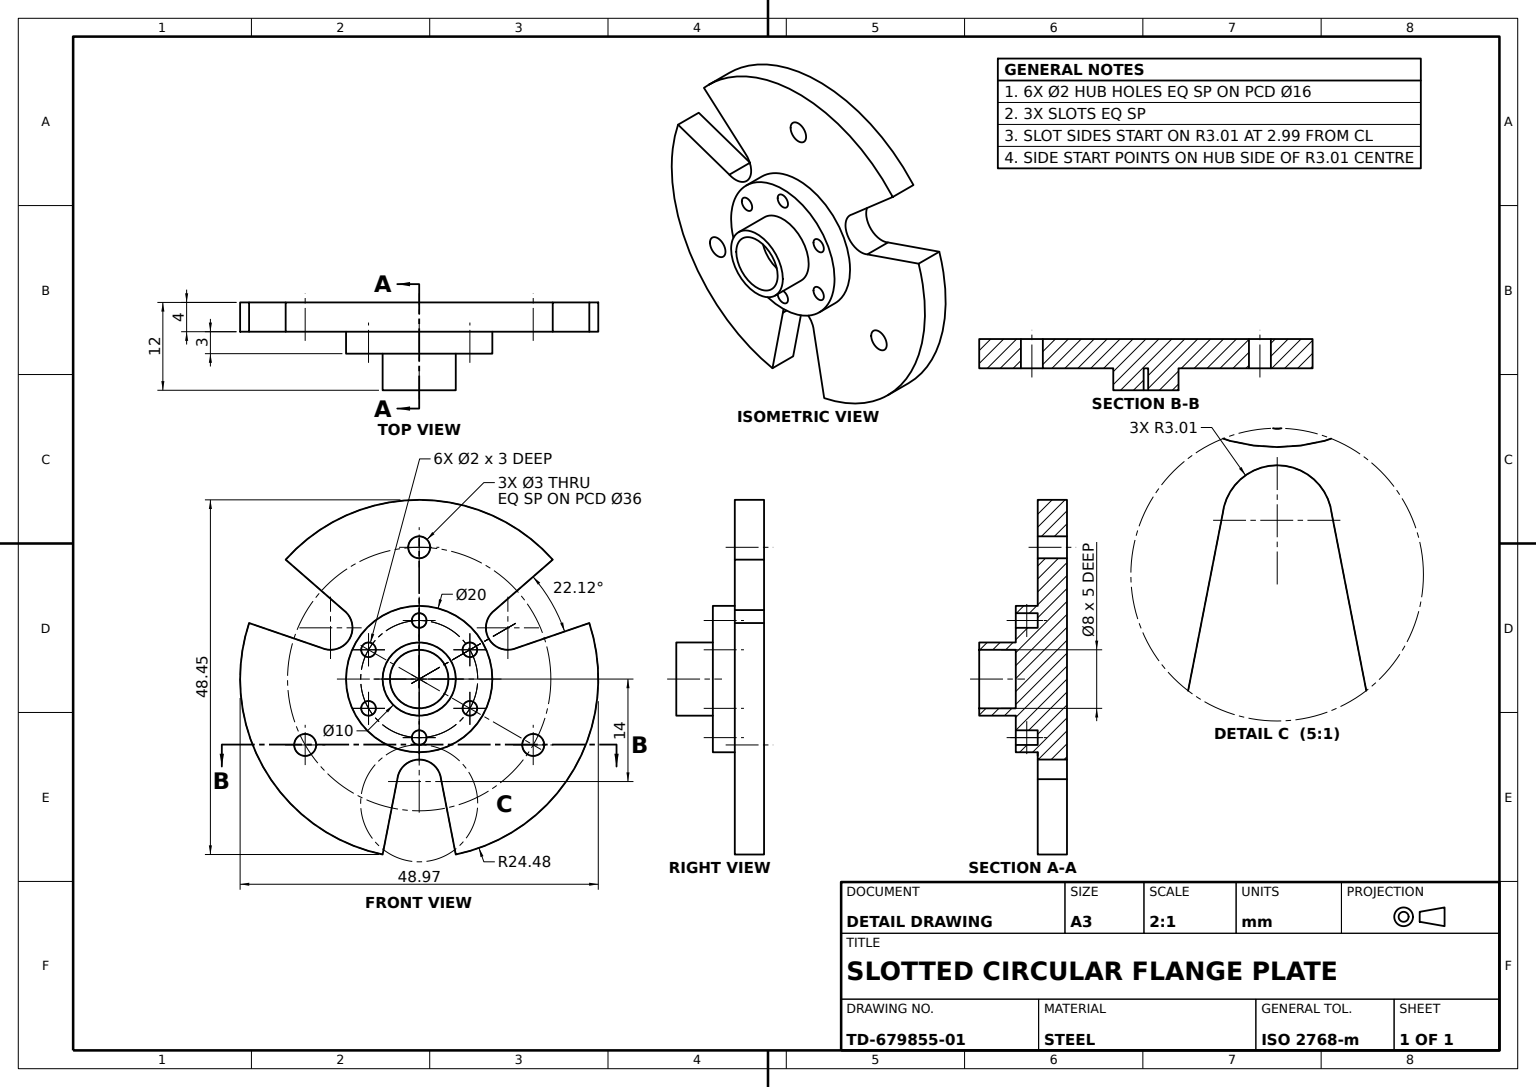
SolidWorks part; units mm, degrees
material "Plain Carbon Steel"
ref_plane "Front Plane" through (0, 0, 0) normal (0, 0, 1) x (1, 0, 0)
ref_plane "Top Plane" through (0, 0, 0) normal (0, 1, 0) x (1, 0, 0)
ref_plane "Right Plane" through (0, 0, 0) normal (1, 0, 0) x (0, 0, -1)
sketch "Flange Plate Sketch" plane through (0, 0, 0) normal (0, 0, 1) x (1, 0, 0)
  line L0 (0, 0) -> (0, 24.4841) construction
  line L1 (0, -17) -> (0, -28.4926) construction
  line L2 (-2.9887, -13.6773) -> (-5, -23.9681)
  line L3 (2.9887, -13.6773) -> (5, -23.9681)
  line L4 (-10.3505, 9.4269) -> (-18.257, 16.3142)
  line L5 (-13.3392, 4.2503) -> (-23.257, 7.6539)
  line L6 (13.3392, 4.2503) -> (23.257, 7.6539)
  line L7 (10.3505, 9.4269) -> (18.257, 16.3142)
  arc A0 (5, -23.9681) -> (23.257, 7.6539) centre (0, 0) ccw
  arc A2 (2.9887, -13.6773) -> (-2.9887, -13.6773) centre (0, -14) ccw
  arc A3 (-13.3392, 4.2503) -> (-10.3505, 9.4269) centre (-12.1244, 7) ccw
  arc A4 (10.3505, 9.4269) -> (13.3392, 4.2503) centre (12.1244, 7) ccw
  arc A5 (-23.257, 7.6539) -> (-5, -23.9681) centre (0, 0) ccw
  arc A6 (18.257, 16.3142) -> (-18.257, 16.3142) centre (0, 0) ccw
  point P13 (0, 0)
  point P25 (0, 0)
  dimension "D1" = 3
  dimension "D4" = 24.4841
  dimension "D5" = 3.0061
  dimension "D6" = 2.9887
  dimension "D7" = 10.3505
  dimension "D2" = 3
  dimension "D3" = 10
extrude "Flange Plate 4mm" add sketch "Flange Plate Sketch" along normal blind 4
sketch "Outer Holes Sketch" plane through (0, 0, 0) normal (0, 0, 1) x (1, 0, 0)
  circle A0 centre (0, 0) radius 18 construction
  circle A1 centre (0, 18) radius 1.5
  circle A2 centre (15.5885, -9) radius 1.5
  circle A3 centre (-15.5885, -9) radius 1.5
  point P11 (0, 0)
  dimension "D1" = 3
  dimension "D2" = 3
  dimension "D5" = 36
extrude "Outer Holes 3x" cut sketch "Outer Holes Sketch" along normal through all
sketch "Hub Sketch" plane through (0, 0, 0) normal (0, 0, 1) x (1, 0, 0)
  circle A0 centre (0, 0) radius 10
  dimension "D1" = 20
extrude "Raised Hub" add sketch "Hub Sketch" along normal blind 7
sketch "Hub Holes Sketch" plane through (0, 0, 7) normal (0, 0, 1) x (1, 0, 0)
  circle A0 centre (0, 0) radius 8 construction
  circle A1 centre (0, 8) radius 1
  circle A2 centre (0.0005, 0.0009) radius 8 construction
  circle A3 centre (6.9287, 4.0009) radius 1
  circle A4 centre (0.0015, 0.0009) radius 8 construction
  circle A5 centre (6.9297, -3.9991) radius 1
  circle A6 centre (0.002, 0) radius 8 construction
  circle A7 centre (0.002, -8) radius 1
  circle A8 centre (0.0015, -0.0009) radius 8 construction
  circle A9 centre (-6.9267, -4.0009) radius 1
  circle A10 centre (0.0005, -0.0009) radius 8 construction
  circle A11 centre (-6.9277, 3.9991) radius 1
  point P27 (0.001, 0)
  dimension "D1" = 6
  dimension "D2" = 16
  dimension "D3" = 2
  dimension "D4" = 0.001
  dimension "D5" = 8
extrude "Hub Holes 6x" cut sketch "Hub Holes Sketch" against normal up to surface (3 mm away) up to face at (10, 0, 4)
sketch "Centre Sleeve Sketch" plane through (0, 0, 7) normal (0, 0, 1) x (1, 0, 0)
  circle A0 centre (0, 0) radius 4
  circle A1 centre (0, 0) radius 5
  dimension "D1" = 1
  dimension "D2" = 8
extrude "Centre Sleeve" add sketch "Centre Sleeve Sketch" along normal blind 5
